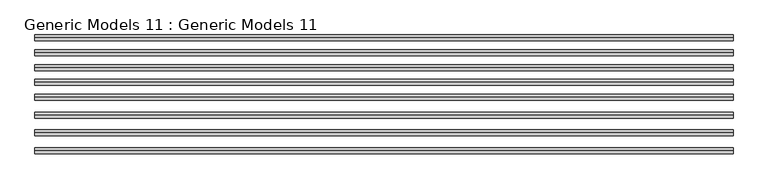
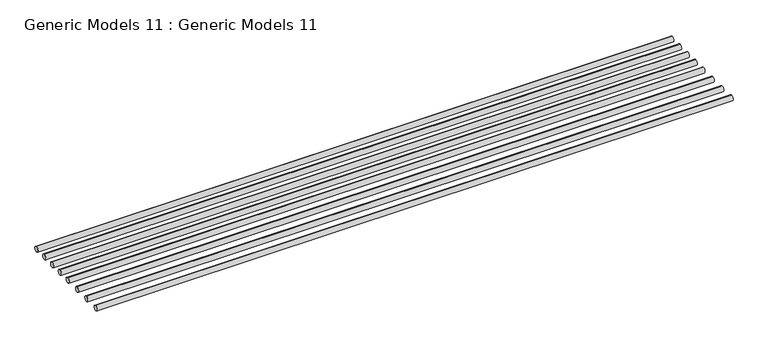
"""IFC4 building model written with IfcOpenShell, lengths in millimetres: proxy geometry, Generic Models 11 : Generic Models 11."""

from ifc_helpers import new_model, si_unit, point, frame, frame_2d, origin, place, context, project, spatial, circle_curve, trimmed, segment, composite_curve, outline, extrude, source, transform, mapped, element, save


def generic_models_11_generic_models_11_8b992ad3(model_context):
    return source(origin(), model_context, "Body", "SweptSolid", [
        extrude(outline(composite_curve([segment(trimmed(circle_curve(frame_2d((-2491.4149754, 10112.1910993)), 25.4), [point((-2491.4149754, 10137.5910993))], [point((-2491.4149754, 10086.7910993))], False, "CARTESIAN"), True, "CONTINUOUS"), segment(trimmed(circle_curve(frame_2d((-2491.4149754, 10112.1910993)), 25.4), [point((-2491.4149754, 10086.7910993))], [point((-2491.4149754, 10137.5910993))], False, "CARTESIAN"), True, "CONTINUOUS")], self_intersect=False)), frame((-10825.2463366, 0.0, 0.0), z_axis=(1.0, 0.0, 0.0), x_axis=(0.0, 1.0, 0.0)), (0.0, 0.0, 1.0), 5970.9487225),
        extrude(outline(composite_curve([segment(trimmed(circle_curve(frame_2d((-2339.0149754, 10112.1910993)), 25.4), [point((-2339.0149754, 10137.5910993))], [point((-2339.0149754, 10086.7910993))], False, "CARTESIAN"), True, "CONTINUOUS"), segment(trimmed(circle_curve(frame_2d((-2339.0149754, 10112.1910993)), 25.4), [point((-2339.0149754, 10086.7910993))], [point((-2339.0149754, 10137.5910993))], False, "CARTESIAN"), True, "CONTINUOUS")], self_intersect=False)), frame((-10825.2463366, 0.0, 0.0), z_axis=(1.0, 0.0, 0.0), x_axis=(0.0, 1.0, 0.0)), (0.0, 0.0, 1.0), 5970.9487225),
        extrude(outline(composite_curve([segment(trimmed(circle_curve(frame_2d((-2186.6149754, 10112.1910993)), 25.4), [point((-2186.6149754, 10137.5910993))], [point((-2186.6149754, 10086.7910993))], False, "CARTESIAN"), True, "CONTINUOUS"), segment(trimmed(circle_curve(frame_2d((-2186.6149754, 10112.1910993)), 25.4), [point((-2186.6149754, 10086.7910993))], [point((-2186.6149754, 10137.5910993))], False, "CARTESIAN"), True, "CONTINUOUS")], self_intersect=False)), frame((-10825.2463366, 0.0, 0.0), z_axis=(1.0, 0.0, 0.0), x_axis=(0.0, 1.0, 0.0)), (0.0, 0.0, 1.0), 5970.9487225),
        extrude(outline(composite_curve([segment(trimmed(circle_curve(frame_2d((-2034.2149754, 10112.1910993)), 25.4), [point((-2034.2149754, 10137.5910993))], [point((-2034.2149754, 10086.7910993))], False, "CARTESIAN"), True, "CONTINUOUS"), segment(trimmed(circle_curve(frame_2d((-2034.2149754, 10112.1910993)), 25.4), [point((-2034.2149754, 10086.7910993))], [point((-2034.2149754, 10137.5910993))], False, "CARTESIAN"), True, "CONTINUOUS")], self_intersect=False)), frame((-10825.2463366, 0.0, 0.0), z_axis=(1.0, 0.0, 0.0), x_axis=(0.0, 1.0, 0.0)), (0.0, 0.0, 1.0), 5970.9487225),
        extrude(outline(composite_curve([segment(trimmed(circle_curve(frame_2d((-1907.2149754, 10112.1910993)), 25.4), [point((-1907.2149754, 10137.5910993))], [point((-1907.2149754, 10086.7910993))], False, "CARTESIAN"), True, "CONTINUOUS"), segment(trimmed(circle_curve(frame_2d((-1907.2149754, 10112.1910993)), 25.4), [point((-1907.2149754, 10086.7910993))], [point((-1907.2149754, 10137.5910993))], False, "CARTESIAN"), True, "CONTINUOUS")], self_intersect=False)), frame((-10825.2463366, 0.0, 0.0), z_axis=(1.0, 0.0, 0.0), x_axis=(0.0, 1.0, 0.0)), (0.0, 0.0, 1.0), 5970.9487225),
        extrude(outline(composite_curve([segment(trimmed(circle_curve(frame_2d((-1780.2149754, 10112.1910993)), 25.4), [point((-1780.2149754, 10137.5910993))], [point((-1780.2149754, 10086.7910993))], False, "CARTESIAN"), True, "CONTINUOUS"), segment(trimmed(circle_curve(frame_2d((-1780.2149754, 10112.1910993)), 25.4), [point((-1780.2149754, 10086.7910993))], [point((-1780.2149754, 10137.5910993))], False, "CARTESIAN"), True, "CONTINUOUS")], self_intersect=False)), frame((-10825.2463366, 0.0, 0.0), z_axis=(1.0, 0.0, 0.0), x_axis=(0.0, 1.0, 0.0)), (0.0, 0.0, 1.0), 5970.9487225),
        extrude(outline(composite_curve([segment(trimmed(circle_curve(frame_2d((-1653.2149754, 10112.1910993)), 25.4), [point((-1653.2149754, 10137.5910993))], [point((-1653.2149754, 10086.7910993))], False, "CARTESIAN"), True, "CONTINUOUS"), segment(trimmed(circle_curve(frame_2d((-1653.2149754, 10112.1910993)), 25.4), [point((-1653.2149754, 10086.7910993))], [point((-1653.2149754, 10137.5910993))], False, "CARTESIAN"), True, "CONTINUOUS")], self_intersect=False)), frame((-10825.2463366, 0.0, 0.0), z_axis=(1.0, 0.0, 0.0), x_axis=(0.0, 1.0, 0.0)), (0.0, 0.0, 1.0), 5970.9487225),
        extrude(outline(composite_curve([segment(trimmed(circle_curve(frame_2d((-1526.2149754, 10112.1910993)), 25.4), [point((-1526.2149754, 10137.5910993))], [point((-1526.2149754, 10086.7910993))], False, "CARTESIAN"), True, "CONTINUOUS"), segment(trimmed(circle_curve(frame_2d((-1526.2149754, 10112.1910993)), 25.4), [point((-1526.2149754, 10086.7910993))], [point((-1526.2149754, 10137.5910993))], False, "CARTESIAN"), True, "CONTINUOUS")], self_intersect=False)), frame((-10825.2463366, 0.0, 0.0), z_axis=(1.0, 0.0, 0.0), x_axis=(0.0, 1.0, 0.0)), (0.0, 0.0, 1.0), 5970.9487225),
    ])


if __name__ == "__main__":
    model = new_model("IFC4")
    model_context = context("Model", 3, world=origin())
    ifc_project = project(units=[si_unit("LENGTHUNIT", "METRE", prefix="MILLI")], contexts=[model_context])
    site = spatial("IfcSite", under=ifc_project)
    building = spatial("IfcBuilding", under=site)
    placement = place(None, origin())
    generic_models_11_generic_models_11_shape = generic_models_11_generic_models_11_8b992ad3(model_context)
    element("IfcBuildingElementProxy", 1, Name="Generic Models 11 : Generic Models 11", ObjectType="Generic Models 11 : Generic Models 11", at=placement, inside=building, context=model_context, shape_type="MappedRepresentation", body=[
        mapped(generic_models_11_generic_models_11_shape, transform((0.0, 0.0, 0.0), x_axis=(1.0, 0.0, 0.0), y_axis=(0.0, 1.0, 0.0), z_axis=(0.0, 0.0, 1.0))),
    ])
    save(model, "model.ifc")
